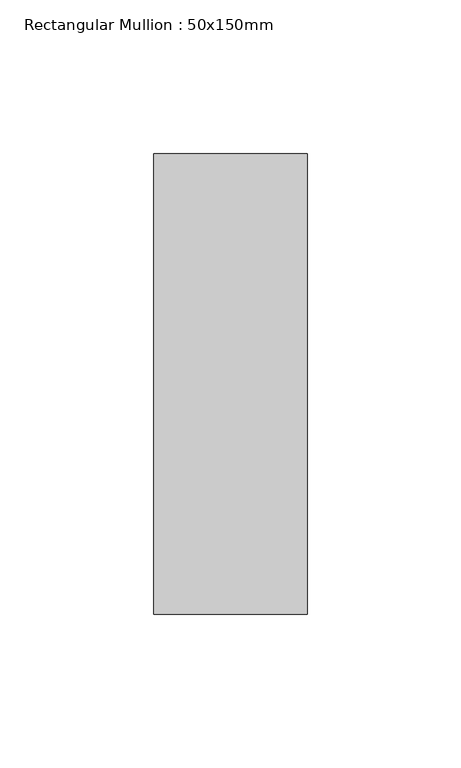
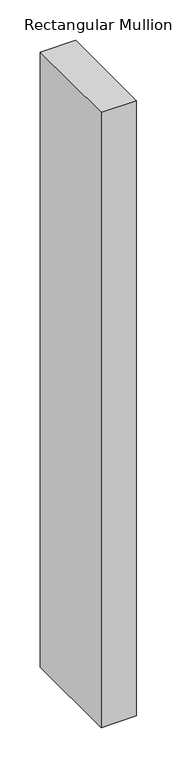
"""IFC4 building model written with IfcOpenShell, lengths in millimetres: member geometry, Rectangular Mullion : 50x150mm."""

from ifc_helpers import new_model, si_unit, frame, origin, place, context, project, spatial, polyline, outline, extrude, source, transform, mapped, element, save


def rectangular_mullion_50x150mm_68afe020(model_context):
    return source(origin(), model_context, "Body", "SweptSolid", [
        extrude(outline(polyline([(0.0, 75.0), (0.0, -75.0), (-50.0, -75.0), (-50.0, 75.0), (0.0, 75.0)])), frame((0.0, 0.0, -927.9), z_axis=(0.0, 0.0, 1.0), x_axis=(1.0, 0.0, 0.0)), (0.0, 0.0, 1.0), 927.9),
    ])


if __name__ == "__main__":
    model = new_model("IFC4")
    model_context = context("Model", 3, world=origin())
    ifc_project = project(units=[si_unit("LENGTHUNIT", "METRE", prefix="MILLI")], contexts=[model_context])
    site = spatial("IfcSite", under=ifc_project)
    building = spatial("IfcBuilding", under=site)
    placement = place(None, origin())
    rectangular_mullion_50x150mm_shape = rectangular_mullion_50x150mm_68afe020(model_context)
    element("IfcMember", 1, ObjectType="Rectangular Mullion : 50x150mm", at=placement, inside=building, context=model_context, shape_type="MappedRepresentation", body=[
        mapped(rectangular_mullion_50x150mm_shape, transform((0.0, 0.0, 0.0), x_axis=(1.0, 0.0, 0.0), y_axis=(0.0, 1.0, 0.0), z_axis=(0.0, 0.0, 1.0))),
    ])
    save(model, "model.ifc")

# Revit data of these elements
# Type "Rectangular Mullion : 50x150mm"
#   Keynote = "H11"
#   built-in parameter 1007304 = 0.492126 (stored number, unit not read)
#   built-in parameter 1007301 = 0.082021 (stored number, unit not read)
#   built-in parameter 1007300 = 0.082021 (stored number, unit not read)
# Element 1 (IfcMember, "Rectangular Mullion : 50x150mm")
#   Materials on its faces: "Aluminium"
# Materials
#   "Aluminium": class "Metal", colour RGB 247 247 247, transparency 0, Description = "Aluminium 6061", Cost = 0
